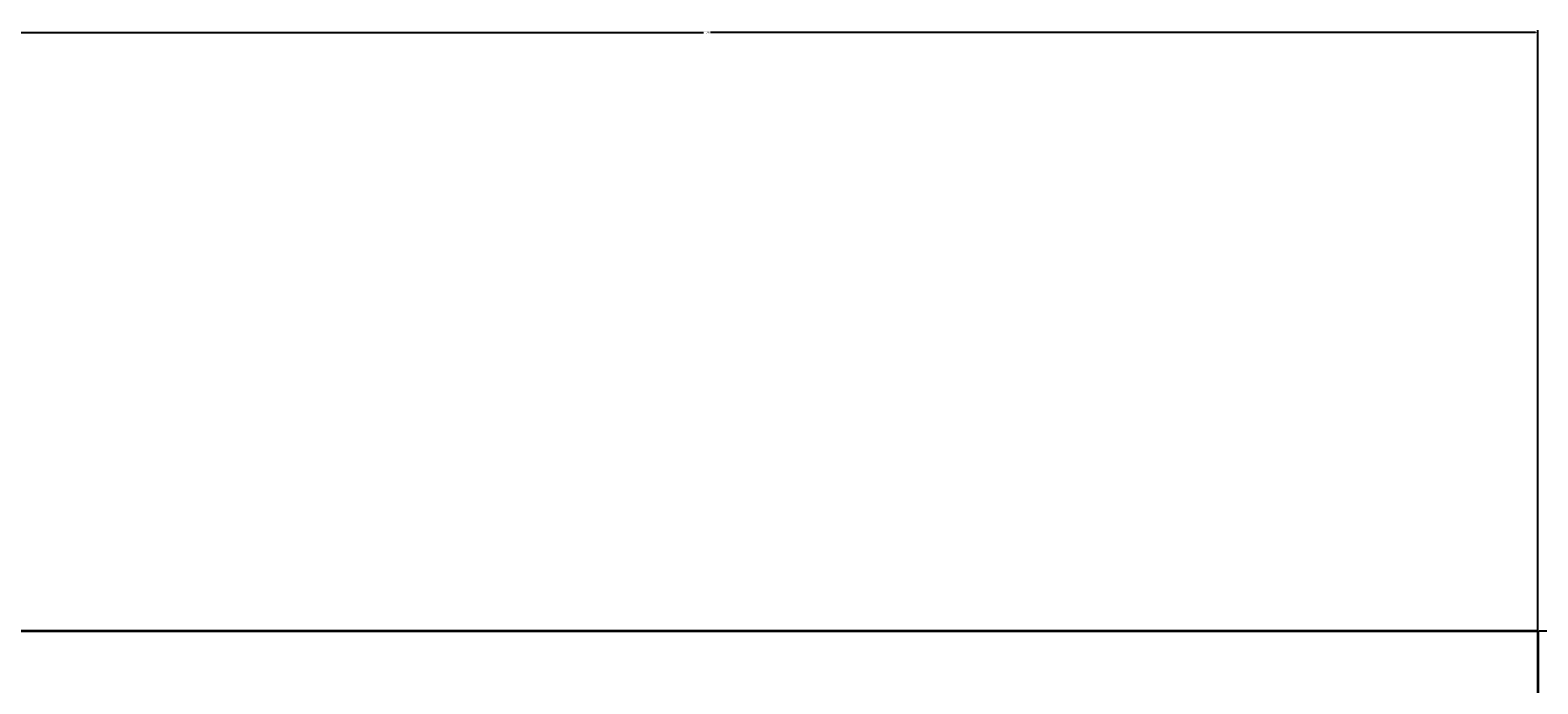
# Model space of a CAD drawing. Units: inches. Extents: x 3731 to 4318, y 1310 to 2388.
# Tile 56 of 57: x 4116 to 4239, y 2334 to 2388. Entities that reach past the tile are written whole.
import ezdxf

# ---------------------------------------------------------------- set-up
doc = ezdxf.new("R2010")
doc.units = ezdxf.units.IN
doc.layers.add('A-ANNO-DIMS', color=2, linetype='Continuous', lineweight=18)
doc.layers.add('A-WALL', color=7, linetype='Continuous', lineweight=35)
doc.styles.get("Standard").update_dxf_attribs({"font": 'arial.ttf'})
doc.dimstyles.get("Standard").update_dxf_attribs({"dimtxt": 0.18, "dimasz": 0.18, "dimexe": 0.18, "dimexo": 0.0625, "dimgap": 0.09, "dimtad": 0, "dimtih": 1, "dimtoh": 1, "dimdec": 4, "dimzin": 0, "dimdsep": 46, "dimtxsty": 'Standard', "dimcen": 0.09, "dimadec": 0, "dimazin": 0, "dimtfac": 1, "dimtdec": 4, "dimtofl": 0, "dimtmove": 0, "dimatfit": 3, "dimfxl": 1, "dimtolj": 1, "dimtzin": 0, "dimarcsym": 0})

# ---------------------------------------------------------------- blocks, each defined once
blk = doc.blocks.new('*D36')
at = {"layer": 'A-ANNO-DIMS', "color": 0, "lineweight": -2, "transparency": 16777216}
for p, q in [((4103.21, 2338.44), (4103.21, 2387.51)), ((4103.39, 2387.33), (4170.93, 2387.33)), ((4239.03, 2387.33), (4171.49, 2387.33)), ((4239.21, 2338.44), (4239.21, 2387.51))]:
    blk.add_line(p, q, dxfattribs=at)
at = {"layer": 'A-ANNO-DIMS', "color": 0, "transparency": 16777216}
for points in [[(4103.39, 2387.36), (4103.39, 2387.3), (4103.21, 2387.33)], [(4239.03, 2387.36), (4239.03, 2387.3), (4239.21, 2387.33)]]:
    blk.add_solid(points, dxfattribs=at)
at = {"layer": 'Defpoints', "color": 0, "transparency": 16777216}
for p in [(4239.21, 2387.33), (4103.21, 2338.38), (4239.21, 2338.38)]:
    blk.add_point(p, dxfattribs=at)
at = {"layer": 'A-ANNO-DIMS', "color": 0, "transparency": 16777216, "insert": (4171.21, 2387.33), "char_height": 0.18, "attachment_point": 5}
blk.add_mtext('\\A1;136', dxfattribs=at)
blk = doc.blocks.new('*D37')
at = {"layer": 'A-ANNO-DIMS', "color": 0, "lineweight": -2, "transparency": 16777216}
for p, q in [((4239.27, 2338.38), (4318.34, 2338.38)), ((4318.16, 2338.2), (4318.16, 2300.56)), ((4318.16, 2262.56), (4318.16, 2300.2)), ((4103.27, 2262.38), (4318.34, 2262.38))]:
    blk.add_line(p, q, dxfattribs=at)
at = {"layer": 'A-ANNO-DIMS', "color": 0, "transparency": 16777216}
for points in [[(4318.13, 2338.2), (4318.19, 2338.2), (4318.16, 2338.38)], [(4318.13, 2262.56), (4318.19, 2262.56), (4318.16, 2262.38)]]:
    blk.add_solid(points, dxfattribs=at)
at = {"layer": 'Defpoints', "color": 0, "transparency": 16777216}
for p in [(4239.21, 2338.38), (4318.16, 2338.38), (4103.21, 2262.38)]:
    blk.add_point(p, dxfattribs=at)
at = {"layer": 'A-ANNO-DIMS', "color": 0, "transparency": 16777216, "insert": (4318.16, 2300.38), "char_height": 0.18, "attachment_point": 5}
blk.add_mtext('\\A1;76', dxfattribs=at)

msp = doc.modelspace()

# ---------------------------------------------------------------- linework, layer by layer
at = {"layer": 'A-WALL'}
for p, q in [((4103.21, 2338.38), (4239.21, 2338.38)), ((4239.21, 2338.38), (4239.21, 1708.38))]:
    msp.add_line(p, q, dxfattribs=at)

# ---------------------------------------------------------------- dimensions: what is measured, and where the dimension line sits
at = {"layer": 'A-ANNO-DIMS'}
dim = msp.add_linear_dim(base=(4239.21, 2387.33), p1=(4103.21, 2338.38), p2=(4239.21, 2338.38), dimstyle='Standard', override={"dimdec": 0, "dimlfac": 1, "dimrnd": 0, "dimzin": 0, "dimdsep": 46, "dimlunit": 2}, dxfattribs=at)
dim.commit()
dim.dimension.update_dxf_attribs({"geometry": '*D36', "text_midpoint": (4171.21, 2387.33)})
dim = msp.add_linear_dim(base=(4318.16, 2338.38), p1=(4103.21, 2262.38), p2=(4239.21, 2338.38), angle=90, dimstyle='Standard', override={"dimdec": 0, "dimlfac": 1, "dimrnd": 0, "dimzin": 0, "dimdsep": 46, "dimlunit": 2}, dxfattribs=at)
dim.commit()
dim.dimension.update_dxf_attribs({"geometry": '*D37', "text_midpoint": (4318.16, 2300.38)})

doc.saveas('drawing.dxf')
